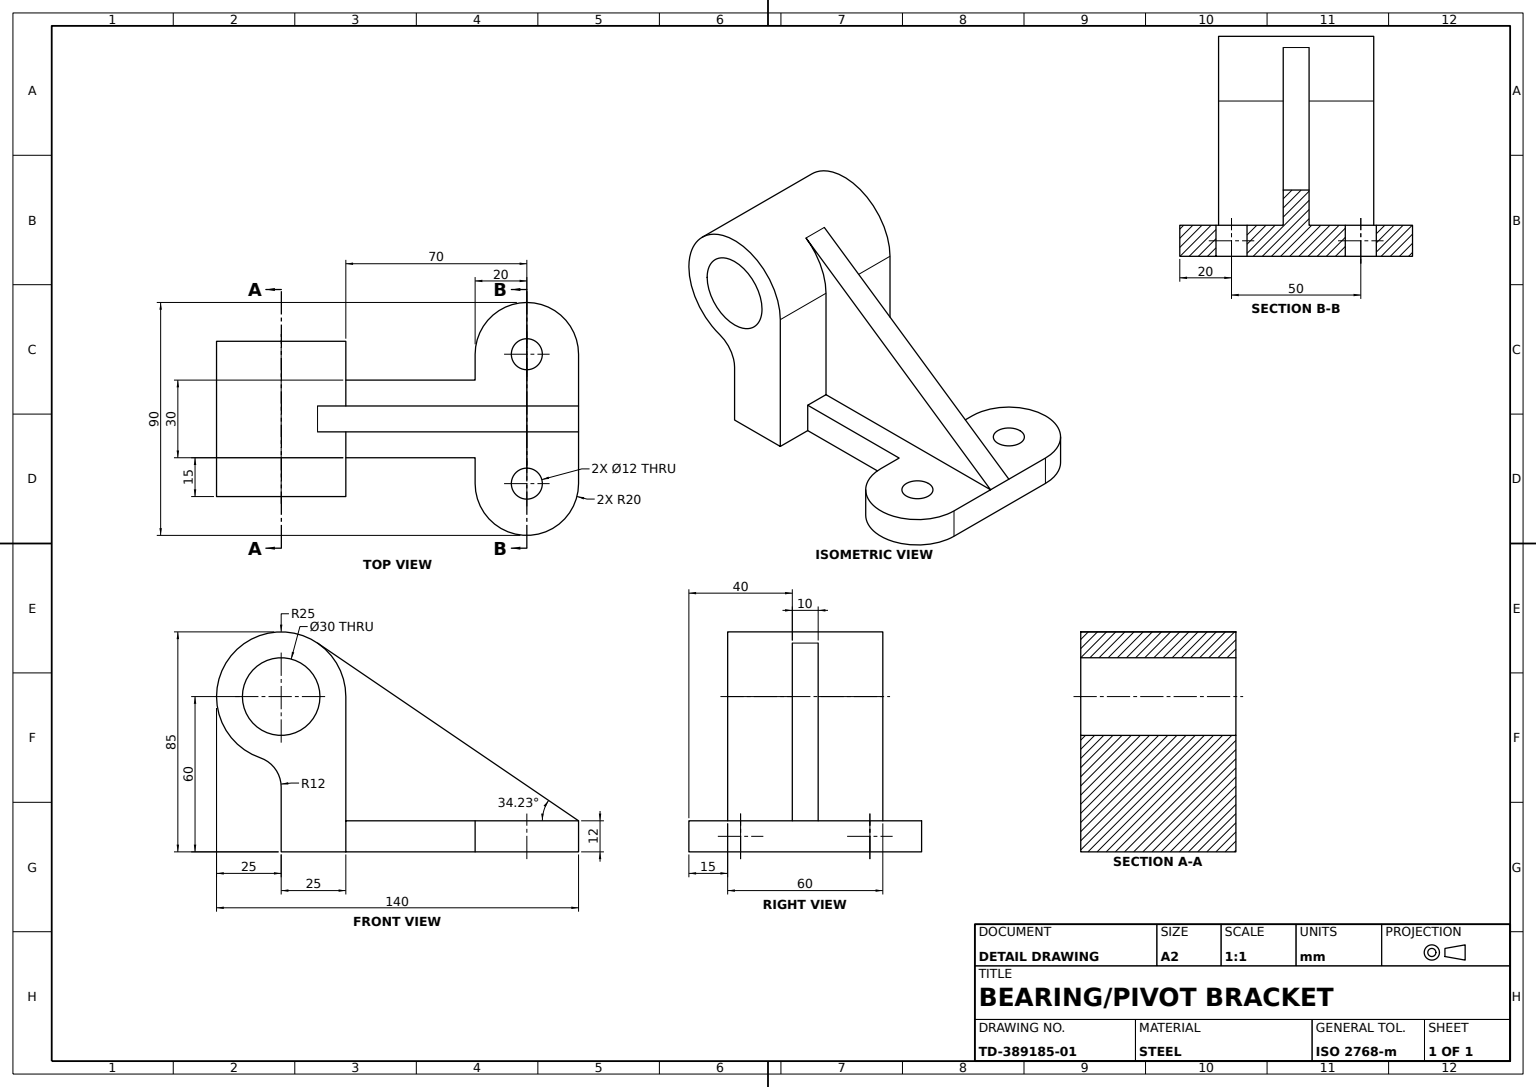
from build123d import *

# Parameters (mm, degrees)
BASE_PLATE_SKETCH_R       = 6
BASE_PLATE_DEPTH          = 6
BEARING_UPRIGHT_SKETCH_R  = 15
BEARING_UPRIGHT_DEPTH     = 30
SUPPORT_RIB_10MM_REACH    = 152.552
SUPPORT_RIB_SKETCH_WALL_W = 425.186572672
SUPPORT_RIB_SKETCH_WALL_H = 10


with BuildPart() as part:
    # Base Plate Sketch → Base Plate (new, symmetric)
    with BuildSketch(Plane(origin=(0, 0, 0), x_dir=(1, 0, 0), z_dir=(0, 1, 0))):
        with BuildLine():
            Line((20, 25), (20, -25))
            ThreePointArc((20, -25), (0, -45), (-20, -25))
            Line((-20, -25), (-20, -15))
            Line((-20, -15), (-70, -15))
            Line((-70, -15), (-70, 15))
            Line((-70, 15), (-20, 15))
            Line((-20, 15), (-20, 25))
            ThreePointArc((-20, 25), (0, 45), (20, 25))
        make_face()
        with Locations(Location((0, 25, 0), (0, 0, 270))):
            Circle(BASE_PLATE_SKETCH_R, mode=Mode.SUBTRACT)
        with Locations(Location((0, -25, 0), (0, 0, 270))):
            Circle(BASE_PLATE_SKETCH_R, mode=Mode.SUBTRACT)
    extrude(amount=BASE_PLATE_DEPTH, both=True)

    # Bearing Upright Sketch → Bearing Upright (add, symmetric)
    with BuildSketch(Plane.XY):
        with BuildLine():
            Line((-70, -6), (-95, -6))
            Line((-95, -6), (-95, 19))
            ThreePointArc((-95, 19), (-97.235198346, 25.974858325), (-103.108108108, 30.351351351))
            ThreePointArc((-103.108108108, 30.351351351), (-109.530954843, 74.34333678), (-70, 54))
            Line((-70, 54), (-70, -6))
        make_face()
        with Locations((-95, 54)):
            Circle(BEARING_UPRIGHT_SKETCH_R, mode=Mode.SUBTRACT)
    extrude(amount=BEARING_UPRIGHT_DEPTH, both=True)

    # Support Rib Sketch wall → Support Rib 10mm (add, up to next)
    with BuildSketch(Plane(origin=(-30.468854155, 40.335036919, 0), x_dir=(-0.826802953509, 0.562491667554, 0), z_dir=(-0.562491667554, -0.826802953509, 0)), mode=Mode.PRIVATE) as support_rib_10mm_sk1:
        Rectangle(SUPPORT_RIB_SKETCH_WALL_W, SUPPORT_RIB_SKETCH_WALL_H)
    support_rib_10mm_tool1 = extrude(support_rib_10mm_sk1.sketch, amount=SUPPORT_RIB_10MM_REACH, mode=Mode.PRIVATE) - part.part
    add(support_rib_10mm_tool1.solids().sort_by_distance((-30.468854155, 40.335036919, 0))[0])


solid = part.part
